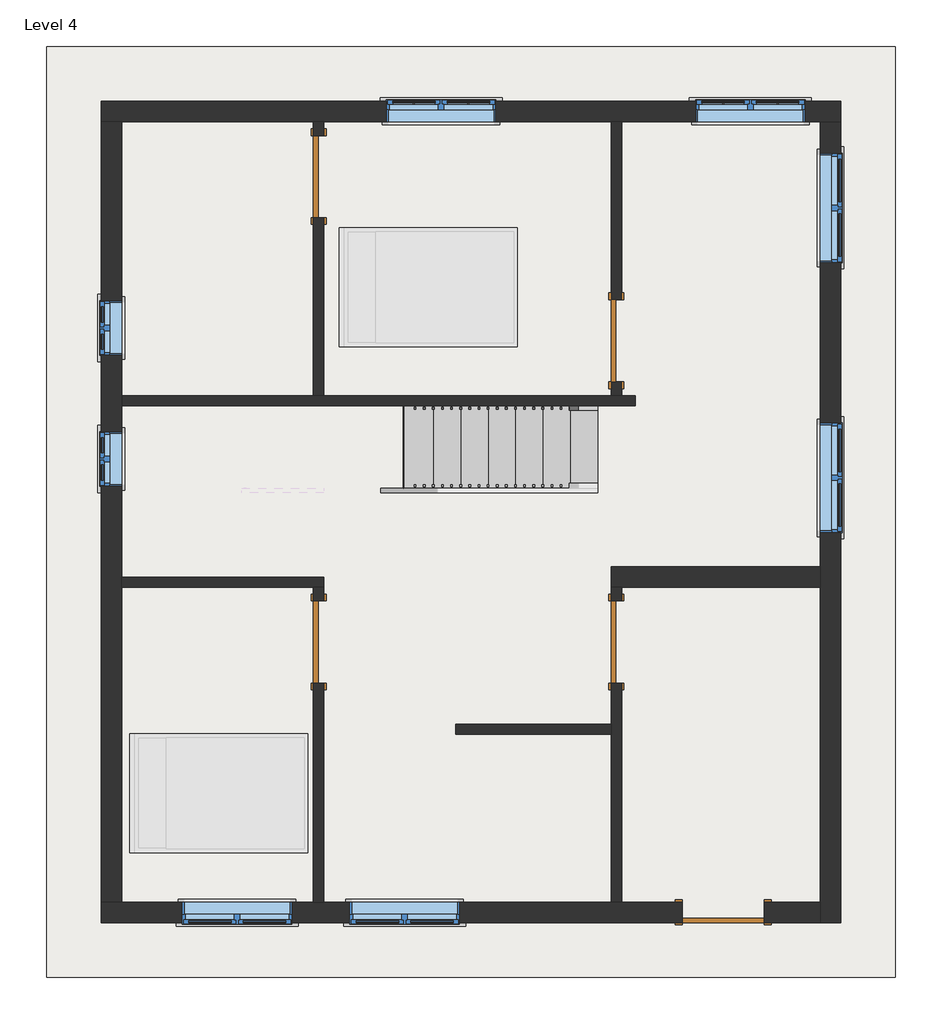
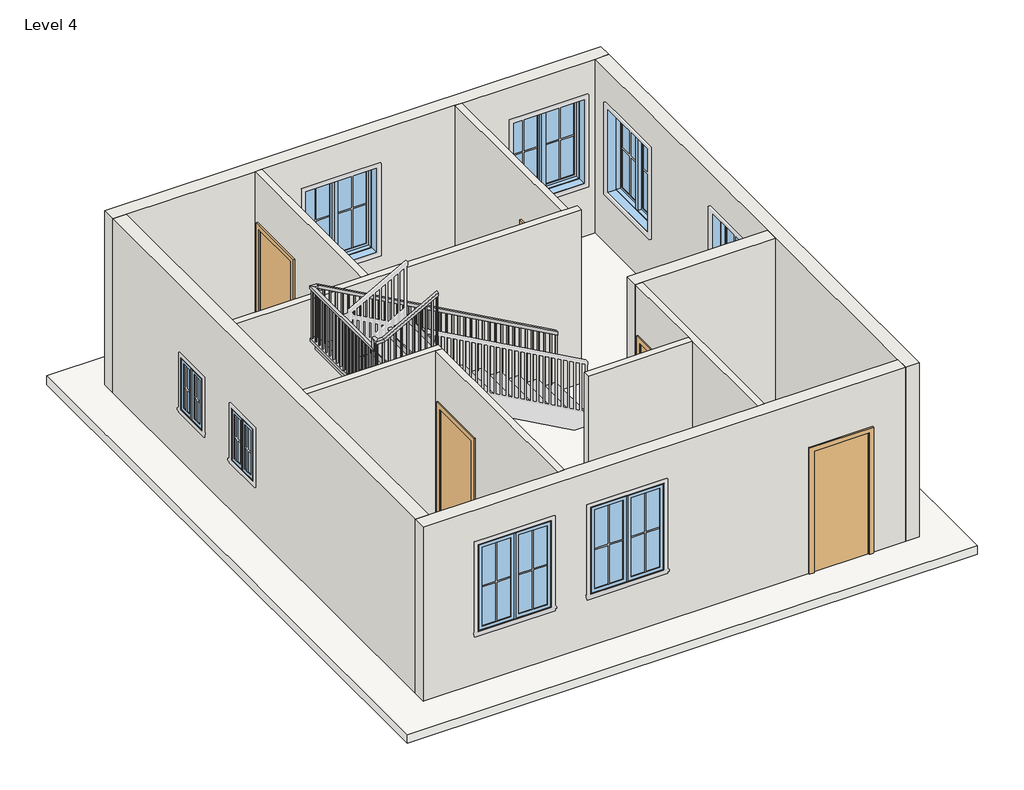
# One storey, part 1 of 2: 12 walls, 8 windows, 5 doors, 1 railing, 1 slab, 1 stair flight.
"""IFC4 building model written with IfcOpenShell, lengths in millimetres."""

from ifc_helpers import new_model, si_unit, frame, origin, place, context, project, spatial, polyline, outline, extrude, faceted_brep, transform, mapped, element, save
from components import door_e5f9f3c4, door_305aa2a5, door_0ca8825f, stair_flight_3eca97f2, window_c417fced, window_8377141f

model = new_model("IFC4")

# Units and contexts
model_context = context("Model", 3, world=origin())
ifc_project = project(units=[si_unit("LENGTHUNIT", "METRE", prefix="MILLI")], contexts=[model_context])

# Site, building, storey
site = spatial("IfcSite", under=ifc_project)
building = spatial("IfcBuilding", under=site)
storey = spatial("IfcBuildingStorey", under=building, Name="Level 4", Elevation=9144.0)

# Doors
placement = place(None, origin())
door_shape = door_e5f9f3c4(model_context)
element("IfcDoor", 1, ObjectType="Single-Flush : 36\" x 84\"", at=placement, inside=storey, context=model_context, shape_type="MappedRepresentation", body=[
    mapped(door_shape, transform((3689.35, 13938.7372886, 9144.0), x_axis=(0.0, 1.0, 0.0), y_axis=(-1.0, 0.0, 0.0), z_axis=(0.0, 0.0, 1.0))),
])
door_2_shape = door_305aa2a5(model_context)
element("IfcDoor", 2, ObjectType="Single-Flush : 36\" x 84\"", at=placement, inside=storey, context=model_context, shape_type="MappedRepresentation", body=[
    mapped(door_2_shape, transform((7004.05, 12109.9372886, 9144.0), x_axis=(0.0, -1.0, 0.0), y_axis=(1.0, 0.0, 0.0), z_axis=(0.0, 0.0, 1.0))),
])
element("IfcDoor", 3, ObjectType="Single-Flush : 36\" x 84\"", at=placement, inside=storey, context=model_context, shape_type="MappedRepresentation", body=[
    mapped(door_2_shape, transform((3689.3519847, 8757.1372886, 9144.0), x_axis=(0.0, -1.0, 0.0), y_axis=(1.0, 0.0, 0.0), z_axis=(0.0, 0.0, 1.0))),
])
element("IfcDoor", 4, ObjectType="Single-Flush : 36\" x 84\"", at=placement, inside=storey, context=model_context, shape_type="MappedRepresentation", body=[
    mapped(door_2_shape, transform((7004.05, 8757.1372886, 9144.0), x_axis=(0.0, -1.0, 0.0), y_axis=(1.0, 0.0, 0.0), z_axis=(0.0, 0.0, 1.0))),
])
door_3_shape = door_0ca8825f(model_context)
element("IfcDoor", 5, ObjectType="Single-Flush : 36\" x 84\"", at=placement, inside=storey, context=model_context, shape_type="MappedRepresentation", body=[
    mapped(door_3_shape, transform((8194.675, 5747.2372886, 9144.0), x_axis=(-1.0, 0.0, 0.0), y_axis=(0.0, -1.0, 0.0), z_axis=(0.0, 0.0, 1.0))),
])

# Railing
element("IfcRailing", 6, ObjectType="Handrail - Rectangular", at=placement, inside=storey, context=model_context, shape_type="SolidModel", body=[
    faceted_brep([(6794.5, 11335.2372886, 10227.7333333), (6794.5, 11335.2372886, 10169.620221), (6794.5, 11386.0372886, 10169.620221), (6794.5, 11386.0372886, 10227.7333333), (2832.1, 11335.2372886, 12429.0666667), (2818.9363978, 11335.2372886, 12378.2666667), (2818.9363978, 11386.0372886, 12378.2666667), (2832.1, 11386.0372886, 12429.0666667), (2768.6, 11335.2372886, 12429.0666667), (2768.6, 11335.2372886, 12378.2666667), (2717.8, 11386.0372886, 12378.2666667), (2717.8, 11386.0372886, 12429.0666667), (2768.6, 9608.0372886, 12429.0666667), (2768.6, 9557.2372886, 12378.2666667), (2717.8, 9557.2372886, 12378.2666667), (2717.8, 9608.0372886, 12429.0666667), (2768.6, 9608.0372886, 12605.4555402), (2768.6, 9557.2372886, 12554.6555402), (2717.8, 9557.2372886, 12554.6555402), (2717.8, 9608.0372886, 12605.4555402), (2768.6, 9531.8372886, 12605.4555402), (2768.6, 9531.8372886, 12554.6555402), (2717.8, 9481.0372886, 12554.6555402), (2717.8, 9481.0372886, 12605.4555402), (2844.8, 9531.8372886, 12605.4555402), (2857.9635773, 9531.8372886, 12554.6555402), (2857.9635773, 9481.0372886, 12554.6555402), (2844.8, 9481.0372886, 12605.4555402), (3746.5019847, 9531.8372886, 13106.4), (3746.5019847, 9481.0372886, 13106.4), (3746.5019847, 9481.0372886, 13048.2869174), (3746.5019847, 9531.8372886, 13048.2869174)], [[[0, 1, 2, 3]], [[1, 0, 4, 5]], [[2, 1, 5, 6]], [[3, 2, 6, 7]], [[0, 3, 7, 4]], [[5, 4, 8, 9]], [[6, 5, 9, 10]], [[7, 6, 10, 11]], [[4, 7, 11, 8]], [[9, 8, 12, 13]], [[10, 9, 13, 14]], [[11, 10, 14, 15]], [[8, 11, 15, 12]], [[13, 12, 16, 17]], [[14, 13, 17, 18]], [[15, 14, 18, 19]], [[12, 15, 19, 16]], [[17, 16, 20, 21]], [[18, 17, 21, 22]], [[19, 18, 22, 23]], [[16, 19, 23, 20]], [[21, 20, 24, 25]], [[22, 21, 25, 26]], [[23, 22, 26, 27]], [[20, 23, 27, 24]], [[28, 29, 30, 31]], [[25, 24, 28, 31]], [[26, 25, 31, 30]], [[27, 26, 30, 29]], [[24, 27, 29, 28]]]),
    extrude(outline(polyline([(13004.1894234, 3667.125), (12993.606113, 3648.075), (12022.6666667, 3648.075), (12022.6666667, 3667.125), (13004.1894234, 3667.125)])), frame((0.0, 9496.9122886, 0.0), z_axis=(0.0, 1.0, 0.0), x_axis=(0.0, 0.0, 1.0)), (0.0, 0.0, 1.0), 19.05),
    extrude(outline(polyline([(12947.7451014, 3565.525), (12937.1617911, 3546.475), (12022.6666667, 3546.475), (12022.6666667, 3565.525), (12947.7451014, 3565.525)])), frame((0.0, 9496.9122886, 0.0), z_axis=(0.0, 1.0, 0.0), x_axis=(0.0, 0.0, 1.0)), (0.0, 0.0, 1.0), 19.05),
    extrude(outline(polyline([(12891.3007795, 3463.925), (12880.7174691, 3444.875), (12022.6666667, 3444.875), (12022.6666667, 3463.925), (12891.3007795, 3463.925)])), frame((0.0, 9496.9122886, 0.0), z_axis=(0.0, 1.0, 0.0), x_axis=(0.0, 0.0, 1.0)), (0.0, 0.0, 1.0), 19.05),
    extrude(outline(polyline([(12834.85609, 3362.325), (12824.2727797, 3343.275), (11853.3333333, 3343.275), (11853.3333333, 3362.325), (12834.85609, 3362.325)])), frame((0.0, 9496.9122886, 0.0), z_axis=(0.0, 1.0, 0.0), x_axis=(0.0, 0.0, 1.0)), (0.0, 0.0, 1.0), 19.05),
    extrude(outline(polyline([(12778.4117681, 3260.725), (12767.8284577, 3241.675), (11853.3333333, 3241.675), (11853.3333333, 3260.725), (12778.4117681, 3260.725)])), frame((0.0, 9496.9122886, 0.0), z_axis=(0.0, 1.0, 0.0), x_axis=(0.0, 0.0, 1.0)), (0.0, 0.0, 1.0), 19.05),
    extrude(outline(polyline([(12721.9674462, 3159.125), (12711.3841358, 3140.075), (11853.3333333, 3140.075), (11853.3333333, 3159.125), (12721.9674462, 3159.125)])), frame((0.0, 9496.9122886, 0.0), z_axis=(0.0, 1.0, 0.0), x_axis=(0.0, 0.0, 1.0)), (0.0, 0.0, 1.0), 19.05),
    extrude(outline(polyline([(12665.5227567, 3057.525), (12654.9394463, 3038.475), (11684.0, 3038.475), (11684.0, 3057.525), (12665.5227567, 3057.525)])), frame((0.0, 9496.9122886, 0.0), z_axis=(0.0, 1.0, 0.0), x_axis=(0.0, 0.0, 1.0)), (0.0, 0.0, 1.0), 19.05),
    extrude(outline(polyline([(12609.0784348, 2955.925), (12598.4951244, 2936.875), (11684.0, 2936.875), (11684.0, 2955.925), (12609.0784348, 2955.925)])), frame((0.0, 9496.9122886, 0.0), z_axis=(0.0, 1.0, 0.0), x_axis=(0.0, 0.0, 1.0)), (0.0, 0.0, 1.0), 19.05),
    extrude(outline(polyline([(12552.6341128, 2854.325), (12542.0508025, 2835.275), (11684.0, 2835.275), (11684.0, 2854.325), (12552.6341128, 2854.325)])), frame((0.0, 9496.9122886, 0.0), z_axis=(0.0, 1.0, 0.0), x_axis=(0.0, 0.0, 1.0)), (0.0, 0.0, 1.0), 19.05),
    extrude(outline(polyline([(2733.675, 9541.3622886), (2752.725, 9541.3622886), (2752.725, 9522.3122886), (2733.675, 9522.3122886), (2733.675, 9541.3622886)])), frame((0.0, 0.0, 11514.6666667), z_axis=(0.0, 0.0, 1.0), x_axis=(1.0, 0.0, 0.0)), (0.0, 0.0, 1.0), 1039.9888736),
    extrude(outline(polyline([(2733.675, 9642.9622886), (2752.725, 9642.9622886), (2752.725, 9623.9122886), (2733.675, 9623.9122886), (2733.675, 9642.9622886)])), frame((0.0, 0.0, 11514.6666667), z_axis=(0.0, 0.0, 1.0), x_axis=(1.0, 0.0, 0.0)), (0.0, 0.0, 1.0), 863.6),
    extrude(outline(polyline([(2733.675, 9744.5622886), (2752.725, 9744.5622886), (2752.725, 9725.5122886), (2733.675, 9725.5122886), (2733.675, 9744.5622886)])), frame((0.0, 0.0, 11514.6666667), z_axis=(0.0, 0.0, 1.0), x_axis=(1.0, 0.0, 0.0)), (0.0, 0.0, 1.0), 863.6),
    extrude(outline(polyline([(2733.675, 9846.1622886), (2752.725, 9846.1622886), (2752.725, 9827.1122886), (2733.675, 9827.1122886), (2733.675, 9846.1622886)])), frame((0.0, 0.0, 11514.6666667), z_axis=(0.0, 0.0, 1.0), x_axis=(1.0, 0.0, 0.0)), (0.0, 0.0, 1.0), 863.6),
    extrude(outline(polyline([(2733.675, 9947.7622886), (2752.725, 9947.7622886), (2752.725, 9928.7122886), (2733.675, 9928.7122886), (2733.675, 9947.7622886)])), frame((0.0, 0.0, 11514.6666667), z_axis=(0.0, 0.0, 1.0), x_axis=(1.0, 0.0, 0.0)), (0.0, 0.0, 1.0), 863.6),
    extrude(outline(polyline([(2733.675, 10049.3622886), (2752.725, 10049.3622886), (2752.725, 10030.3122886), (2733.675, 10030.3122886), (2733.675, 10049.3622886)])), frame((0.0, 0.0, 11514.6666667), z_axis=(0.0, 0.0, 1.0), x_axis=(1.0, 0.0, 0.0)), (0.0, 0.0, 1.0), 863.6),
    extrude(outline(polyline([(2733.675, 10150.9622886), (2752.725, 10150.9622886), (2752.725, 10131.9122886), (2733.675, 10131.9122886), (2733.675, 10150.9622886)])), frame((0.0, 0.0, 11514.6666667), z_axis=(0.0, 0.0, 1.0), x_axis=(1.0, 0.0, 0.0)), (0.0, 0.0, 1.0), 863.6),
    extrude(outline(polyline([(2733.675, 10252.5622886), (2752.725, 10252.5622886), (2752.725, 10233.5122886), (2733.675, 10233.5122886), (2733.675, 10252.5622886)])), frame((0.0, 0.0, 11514.6666667), z_axis=(0.0, 0.0, 1.0), x_axis=(1.0, 0.0, 0.0)), (0.0, 0.0, 1.0), 863.6),
    extrude(outline(polyline([(2733.675, 10354.1622886), (2752.725, 10354.1622886), (2752.725, 10335.1122886), (2733.675, 10335.1122886), (2733.675, 10354.1622886)])), frame((0.0, 0.0, 11514.6666667), z_axis=(0.0, 0.0, 1.0), x_axis=(1.0, 0.0, 0.0)), (0.0, 0.0, 1.0), 863.6),
    extrude(outline(polyline([(2733.675, 10455.7622886), (2752.725, 10455.7622886), (2752.725, 10436.7122886), (2733.675, 10436.7122886), (2733.675, 10455.7622886)])), frame((0.0, 0.0, 11514.6666667), z_axis=(0.0, 0.0, 1.0), x_axis=(1.0, 0.0, 0.0)), (0.0, 0.0, 1.0), 863.6),
    extrude(outline(polyline([(2733.675, 10557.3622886), (2752.725, 10557.3622886), (2752.725, 10538.3122886), (2733.675, 10538.3122886), (2733.675, 10557.3622886)])), frame((0.0, 0.0, 11514.6666667), z_axis=(0.0, 0.0, 1.0), x_axis=(1.0, 0.0, 0.0)), (0.0, 0.0, 1.0), 863.6),
    extrude(outline(polyline([(2733.675, 10658.9622886), (2752.725, 10658.9622886), (2752.725, 10639.9122886), (2733.675, 10639.9122886), (2733.675, 10658.9622886)])), frame((0.0, 0.0, 11514.6666667), z_axis=(0.0, 0.0, 1.0), x_axis=(1.0, 0.0, 0.0)), (0.0, 0.0, 1.0), 863.6),
    extrude(outline(polyline([(2733.675, 10760.5622886), (2752.725, 10760.5622886), (2752.725, 10741.5122886), (2733.675, 10741.5122886), (2733.675, 10760.5622886)])), frame((0.0, 0.0, 11514.6666667), z_axis=(0.0, 0.0, 1.0), x_axis=(1.0, 0.0, 0.0)), (0.0, 0.0, 1.0), 863.6),
    extrude(outline(polyline([(2733.675, 10862.1622886), (2752.725, 10862.1622886), (2752.725, 10843.1122886), (2733.675, 10843.1122886), (2733.675, 10862.1622886)])), frame((0.0, 0.0, 11514.6666667), z_axis=(0.0, 0.0, 1.0), x_axis=(1.0, 0.0, 0.0)), (0.0, 0.0, 1.0), 863.6),
    extrude(outline(polyline([(2733.675, 10963.7622886), (2752.725, 10963.7622886), (2752.725, 10944.7122886), (2733.675, 10944.7122886), (2733.675, 10963.7622886)])), frame((0.0, 0.0, 11514.6666667), z_axis=(0.0, 0.0, 1.0), x_axis=(1.0, 0.0, 0.0)), (0.0, 0.0, 1.0), 863.6),
    extrude(outline(polyline([(2733.675, 11065.3622886), (2752.725, 11065.3622886), (2752.725, 11046.3122886), (2733.675, 11046.3122886), (2733.675, 11065.3622886)])), frame((0.0, 0.0, 11514.6666667), z_axis=(0.0, 0.0, 1.0), x_axis=(1.0, 0.0, 0.0)), (0.0, 0.0, 1.0), 863.6),
    extrude(outline(polyline([(2733.675, 11166.9622886), (2752.725, 11166.9622886), (2752.725, 11147.9122886), (2733.675, 11147.9122886), (2733.675, 11166.9622886)])), frame((0.0, 0.0, 11514.6666667), z_axis=(0.0, 0.0, 1.0), x_axis=(1.0, 0.0, 0.0)), (0.0, 0.0, 1.0), 863.6),
    extrude(outline(polyline([(2733.675, 11268.5622886), (2752.725, 11268.5622886), (2752.725, 11249.5122886), (2733.675, 11249.5122886), (2733.675, 11268.5622886)])), frame((0.0, 0.0, 11514.6666667), z_axis=(0.0, 0.0, 1.0), x_axis=(1.0, 0.0, 0.0)), (0.0, 0.0, 1.0), 863.6),
    extrude(outline(polyline([(12365.6618876, 2841.625), (12376.245221, 2822.575), (11514.6666667, 2822.575), (11514.6666667, 2841.625), (12365.6618876, 2841.625)])), frame((0.0, 11351.1122886, 0.0), z_axis=(0.0, 1.0, 0.0), x_axis=(0.0, 0.0, 1.0)), (0.0, 0.0, 1.0), 19.05),
    extrude(outline(polyline([(12309.2174432, 2943.225), (12319.8007765, 2924.175), (11345.3333333, 2924.175), (11345.3333333, 2943.225), (12309.2174432, 2943.225)])), frame((0.0, 11351.1122886, 0.0), z_axis=(0.0, 1.0, 0.0), x_axis=(0.0, 0.0, 1.0)), (0.0, 0.0, 1.0), 19.05),
    extrude(outline(polyline([(12252.7729988, 3044.825), (12263.3563321, 3025.775), (11345.3333333, 3025.775), (11345.3333333, 3044.825), (12252.7729988, 3044.825)])), frame((0.0, 11351.1122886, 0.0), z_axis=(0.0, 1.0, 0.0), x_axis=(0.0, 0.0, 1.0)), (0.0, 0.0, 1.0), 19.05),
    extrude(outline(polyline([(12196.3285543, 3146.425), (12206.9118876, 3127.375), (11345.3333333, 3127.375), (11345.3333333, 3146.425), (12196.3285543, 3146.425)])), frame((0.0, 11351.1122886, 0.0), z_axis=(0.0, 1.0, 0.0), x_axis=(0.0, 0.0, 1.0)), (0.0, 0.0, 1.0), 19.05),
    extrude(outline(polyline([(12139.8841099, 3248.025), (12150.4674432, 3228.975), (11176.0, 3228.975), (11176.0, 3248.025), (12139.8841099, 3248.025)])), frame((0.0, 11351.1122886, 0.0), z_axis=(0.0, 1.0, 0.0), x_axis=(0.0, 0.0, 1.0)), (0.0, 0.0, 1.0), 19.05),
    extrude(outline(polyline([(12083.4396654, 3349.625), (12094.0229988, 3330.575), (11176.0, 3330.575), (11176.0, 3349.625), (12083.4396654, 3349.625)])), frame((0.0, 11351.1122886, 0.0), z_axis=(0.0, 1.0, 0.0), x_axis=(0.0, 0.0, 1.0)), (0.0, 0.0, 1.0), 19.05),
    extrude(outline(polyline([(12026.995221, 3451.225), (12037.5785543, 3432.175), (11176.0, 3432.175), (11176.0, 3451.225), (12026.995221, 3451.225)])), frame((0.0, 11351.1122886, 0.0), z_axis=(0.0, 1.0, 0.0), x_axis=(0.0, 0.0, 1.0)), (0.0, 0.0, 1.0), 19.05),
    extrude(outline(polyline([(11970.5507765, 3552.825), (11981.1341099, 3533.775), (11006.6666667, 3533.775), (11006.6666667, 3552.825), (11970.5507765, 3552.825)])), frame((0.0, 11351.1122886, 0.0), z_axis=(0.0, 1.0, 0.0), x_axis=(0.0, 0.0, 1.0)), (0.0, 0.0, 1.0), 19.05),
    extrude(outline(polyline([(11914.1063321, 3654.425), (11924.6896654, 3635.375), (11006.6666667, 3635.375), (11006.6666667, 3654.425), (11914.1063321, 3654.425)])), frame((0.0, 11351.1122886, 0.0), z_axis=(0.0, 1.0, 0.0), x_axis=(0.0, 0.0, 1.0)), (0.0, 0.0, 1.0), 19.05),
    extrude(outline(polyline([(11857.6618876, 3756.025), (11868.245221, 3736.975), (11006.6666667, 3736.975), (11006.6666667, 3756.025), (11857.6618876, 3756.025)])), frame((0.0, 11351.1122886, 0.0), z_axis=(0.0, 1.0, 0.0), x_axis=(0.0, 0.0, 1.0)), (0.0, 0.0, 1.0), 19.05),
    extrude(outline(polyline([(11801.2174432, 3857.625), (11811.8007765, 3838.575), (10837.3333333, 3838.575), (10837.3333333, 3857.625), (11801.2174432, 3857.625)])), frame((0.0, 11351.1122886, 0.0), z_axis=(0.0, 1.0, 0.0), x_axis=(0.0, 0.0, 1.0)), (0.0, 0.0, 1.0), 19.05),
    extrude(outline(polyline([(11744.7729988, 3959.225), (11755.3563321, 3940.175), (10837.3333333, 3940.175), (10837.3333333, 3959.225), (11744.7729988, 3959.225)])), frame((0.0, 11351.1122886, 0.0), z_axis=(0.0, 1.0, 0.0), x_axis=(0.0, 0.0, 1.0)), (0.0, 0.0, 1.0), 19.05),
    extrude(outline(polyline([(11688.3285543, 4060.825), (11698.9118876, 4041.775), (10837.3333333, 4041.775), (10837.3333333, 4060.825), (11688.3285543, 4060.825)])), frame((0.0, 11351.1122886, 0.0), z_axis=(0.0, 1.0, 0.0), x_axis=(0.0, 0.0, 1.0)), (0.0, 0.0, 1.0), 19.05),
    extrude(outline(polyline([(11631.8841099, 4162.425), (11642.4674432, 4143.375), (10668.0, 4143.375), (10668.0, 4162.425), (11631.8841099, 4162.425)])), frame((0.0, 11351.1122886, 0.0), z_axis=(0.0, 1.0, 0.0), x_axis=(0.0, 0.0, 1.0)), (0.0, 0.0, 1.0), 19.05),
    extrude(outline(polyline([(11575.4396654, 4264.025), (11586.0229988, 4244.975), (10668.0, 4244.975), (10668.0, 4264.025), (11575.4396654, 4264.025)])), frame((0.0, 11351.1122886, 0.0), z_axis=(0.0, 1.0, 0.0), x_axis=(0.0, 0.0, 1.0)), (0.0, 0.0, 1.0), 19.05),
    extrude(outline(polyline([(11518.995221, 4365.625), (11529.5785543, 4346.575), (10668.0, 4346.575), (10668.0, 4365.625), (11518.995221, 4365.625)])), frame((0.0, 11351.1122886, 0.0), z_axis=(0.0, 1.0, 0.0), x_axis=(0.0, 0.0, 1.0)), (0.0, 0.0, 1.0), 19.05),
    extrude(outline(polyline([(11462.5507765, 4467.225), (11473.1341099, 4448.175), (10498.6666667, 4448.175), (10498.6666667, 4467.225), (11462.5507765, 4467.225)])), frame((0.0, 11351.1122886, 0.0), z_axis=(0.0, 1.0, 0.0), x_axis=(0.0, 0.0, 1.0)), (0.0, 0.0, 1.0), 19.05),
    extrude(outline(polyline([(11406.1063321, 4568.825), (11416.6896654, 4549.775), (10498.6666667, 4549.775), (10498.6666667, 4568.825), (11406.1063321, 4568.825)])), frame((0.0, 11351.1122886, 0.0), z_axis=(0.0, 1.0, 0.0), x_axis=(0.0, 0.0, 1.0)), (0.0, 0.0, 1.0), 19.05),
    extrude(outline(polyline([(11349.6618876, 4670.425), (11360.245221, 4651.375), (10498.6666667, 4651.375), (10498.6666667, 4670.425), (11349.6618876, 4670.425)])), frame((0.0, 11351.1122886, 0.0), z_axis=(0.0, 1.0, 0.0), x_axis=(0.0, 0.0, 1.0)), (0.0, 0.0, 1.0), 19.05),
    extrude(outline(polyline([(11293.2174432, 4772.025), (11303.8007765, 4752.975), (10329.3333333, 4752.975), (10329.3333333, 4772.025), (11293.2174432, 4772.025)])), frame((0.0, 11351.1122886, 0.0), z_axis=(0.0, 1.0, 0.0), x_axis=(0.0, 0.0, 1.0)), (0.0, 0.0, 1.0), 19.05),
    extrude(outline(polyline([(11236.7729988, 4873.625), (11247.3563321, 4854.575), (10329.3333333, 4854.575), (10329.3333333, 4873.625), (11236.7729988, 4873.625)])), frame((0.0, 11351.1122886, 0.0), z_axis=(0.0, 1.0, 0.0), x_axis=(0.0, 0.0, 1.0)), (0.0, 0.0, 1.0), 19.05),
    extrude(outline(polyline([(11180.3285543, 4975.225), (11190.9118876, 4956.175), (10329.3333333, 4956.175), (10329.3333333, 4975.225), (11180.3285543, 4975.225)])), frame((0.0, 11351.1122886, 0.0), z_axis=(0.0, 1.0, 0.0), x_axis=(0.0, 0.0, 1.0)), (0.0, 0.0, 1.0), 19.05),
    extrude(outline(polyline([(11123.8841099, 5076.825), (11134.4674432, 5057.775), (10160.0, 5057.775), (10160.0, 5076.825), (11123.8841099, 5076.825)])), frame((0.0, 11351.1122886, 0.0), z_axis=(0.0, 1.0, 0.0), x_axis=(0.0, 0.0, 1.0)), (0.0, 0.0, 1.0), 19.05),
    extrude(outline(polyline([(11067.4396654, 5178.425), (11078.0229988, 5159.375), (10160.0, 5159.375), (10160.0, 5178.425), (11067.4396654, 5178.425)])), frame((0.0, 11351.1122886, 0.0), z_axis=(0.0, 1.0, 0.0), x_axis=(0.0, 0.0, 1.0)), (0.0, 0.0, 1.0), 19.05),
    extrude(outline(polyline([(11010.995221, 5280.025), (11021.5785543, 5260.975), (10160.0, 5260.975), (10160.0, 5280.025), (11010.995221, 5280.025)])), frame((0.0, 11351.1122886, 0.0), z_axis=(0.0, 1.0, 0.0), x_axis=(0.0, 0.0, 1.0)), (0.0, 0.0, 1.0), 19.05),
    extrude(outline(polyline([(10954.5507765, 5381.625), (10965.1341099, 5362.575), (9990.6666667, 5362.575), (9990.6666667, 5381.625), (10954.5507765, 5381.625)])), frame((0.0, 11351.1122886, 0.0), z_axis=(0.0, 1.0, 0.0), x_axis=(0.0, 0.0, 1.0)), (0.0, 0.0, 1.0), 19.05),
    extrude(outline(polyline([(10898.1063321, 5483.225), (10908.6896654, 5464.175), (9990.6666667, 5464.175), (9990.6666667, 5483.225), (10898.1063321, 5483.225)])), frame((0.0, 11351.1122886, 0.0), z_axis=(0.0, 1.0, 0.0), x_axis=(0.0, 0.0, 1.0)), (0.0, 0.0, 1.0), 19.05),
    extrude(outline(polyline([(10841.6618876, 5584.825), (10852.245221, 5565.775), (9990.6666667, 5565.775), (9990.6666667, 5584.825), (10841.6618876, 5584.825)])), frame((0.0, 11351.1122886, 0.0), z_axis=(0.0, 1.0, 0.0), x_axis=(0.0, 0.0, 1.0)), (0.0, 0.0, 1.0), 19.05),
    extrude(outline(polyline([(10785.2174432, 5686.425), (10795.8007765, 5667.375), (9821.3333333, 5667.375), (9821.3333333, 5686.425), (10785.2174432, 5686.425)])), frame((0.0, 11351.1122886, 0.0), z_axis=(0.0, 1.0, 0.0), x_axis=(0.0, 0.0, 1.0)), (0.0, 0.0, 1.0), 19.05),
    extrude(outline(polyline([(10728.7729988, 5788.025), (10739.3563321, 5768.975), (9821.3333333, 5768.975), (9821.3333333, 5788.025), (10728.7729988, 5788.025)])), frame((0.0, 11351.1122886, 0.0), z_axis=(0.0, 1.0, 0.0), x_axis=(0.0, 0.0, 1.0)), (0.0, 0.0, 1.0), 19.05),
    extrude(outline(polyline([(10672.3285543, 5889.625), (10682.9118876, 5870.575), (9821.3333333, 5870.575), (9821.3333333, 5889.625), (10672.3285543, 5889.625)])), frame((0.0, 11351.1122886, 0.0), z_axis=(0.0, 1.0, 0.0), x_axis=(0.0, 0.0, 1.0)), (0.0, 0.0, 1.0), 19.05),
    extrude(outline(polyline([(10615.8841099, 5991.225), (10626.4674432, 5972.175), (9652.0, 5972.175), (9652.0, 5991.225), (10615.8841099, 5991.225)])), frame((0.0, 11351.1122886, 0.0), z_axis=(0.0, 1.0, 0.0), x_axis=(0.0, 0.0, 1.0)), (0.0, 0.0, 1.0), 19.05),
    extrude(outline(polyline([(10559.4396654, 6092.825), (10570.0229988, 6073.775), (9652.0, 6073.775), (9652.0, 6092.825), (10559.4396654, 6092.825)])), frame((0.0, 11351.1122886, 0.0), z_axis=(0.0, 1.0, 0.0), x_axis=(0.0, 0.0, 1.0)), (0.0, 0.0, 1.0), 19.05),
    extrude(outline(polyline([(10502.995221, 6194.425), (10513.5785543, 6175.375), (9652.0, 6175.375), (9652.0, 6194.425), (10502.995221, 6194.425)])), frame((0.0, 11351.1122886, 0.0), z_axis=(0.0, 1.0, 0.0), x_axis=(0.0, 0.0, 1.0)), (0.0, 0.0, 1.0), 19.05),
    extrude(outline(polyline([(10446.5507765, 6296.025), (10457.1341099, 6276.975), (9482.6666667, 6276.975), (9482.6666667, 6296.025), (10446.5507765, 6296.025)])), frame((0.0, 11351.1122886, 0.0), z_axis=(0.0, 1.0, 0.0), x_axis=(0.0, 0.0, 1.0)), (0.0, 0.0, 1.0), 19.05),
    extrude(outline(polyline([(10390.1063321, 6397.625), (10400.6896654, 6378.575), (9482.6666667, 6378.575), (9482.6666667, 6397.625), (10390.1063321, 6397.625)])), frame((0.0, 11351.1122886, 0.0), z_axis=(0.0, 1.0, 0.0), x_axis=(0.0, 0.0, 1.0)), (0.0, 0.0, 1.0), 19.05),
    extrude(outline(polyline([(10333.6618876, 6499.225), (10344.245221, 6480.175), (9482.6666667, 6480.175), (9482.6666667, 6499.225), (10333.6618876, 6499.225)])), frame((0.0, 11351.1122886, 0.0), z_axis=(0.0, 1.0, 0.0), x_axis=(0.0, 0.0, 1.0)), (0.0, 0.0, 1.0), 19.05),
    extrude(outline(polyline([(10277.2174432, 6600.825), (10287.8007765, 6581.775), (9313.3333333, 6581.775), (9313.3333333, 6600.825), (10277.2174432, 6600.825)])), frame((0.0, 11351.1122886, 0.0), z_axis=(0.0, 1.0, 0.0), x_axis=(0.0, 0.0, 1.0)), (0.0, 0.0, 1.0), 19.05),
    extrude(outline(polyline([(10220.7729988, 6702.425), (10231.3563321, 6683.375), (9313.3333333, 6683.375), (9313.3333333, 6702.425), (10220.7729988, 6702.425)])), frame((0.0, 11351.1122886, 0.0), z_axis=(0.0, 1.0, 0.0), x_axis=(0.0, 0.0, 1.0)), (0.0, 0.0, 1.0), 19.05),
    extrude(outline(polyline([(2733.675, 9515.9622886), (2752.725, 9515.9622886), (2752.725, 9496.9122886), (2733.675, 9496.9122886), (2733.675, 9515.9622886)])), frame((0.0, 0.0, 11514.6666667), z_axis=(0.0, 0.0, 1.0), x_axis=(1.0, 0.0, 0.0)), (0.0, 0.0, 1.0), 1039.9888736),
    extrude(outline(polyline([(2752.725, 11370.1622886), (2752.725, 11351.1122886), (2733.675, 11351.1122886), (2733.675, 11370.1622886), (2752.725, 11370.1622886)])), frame((0.0, 0.0, 11514.6666667), z_axis=(0.0, 0.0, 1.0), x_axis=(1.0, 0.0, 0.0)), (0.0, 0.0, 1.0), 863.6),
    extrude(outline(polyline([(13048.2869174, 3746.5019847), (13037.703607, 3727.4519847), (12022.6666667, 3727.4519847), (12022.6666667, 3746.5019847), (13048.2869174, 3746.5019847)])), frame((0.0, 9496.9122886, 0.0), z_axis=(0.0, 1.0, 0.0), x_axis=(0.0, 0.0, 1.0)), (0.0, 0.0, 1.0), 19.05),
    extrude(outline(polyline([(10169.620221, 6794.5), (10180.2035543, 6775.45), (9313.3333333, 6775.45), (9313.3333333, 6794.5), (10169.620221, 6794.5)])), frame((0.0, 11351.1122886, 0.0), z_axis=(0.0, 1.0, 0.0), x_axis=(0.0, 0.0, 1.0)), (0.0, 0.0, 1.0), 19.05),
])

# Slab
element("IfcSlab", 7, ObjectType="Generic - 12\"", at=placement, inside=storey, context=model_context, shape_type="SweptSolid", body=[
    extrude(outline(polyline([(10109.2, 15386.5372886), (10109.2, 5023.3372886), (660.4, 5023.3372886), (660.4, 15386.5372886), (10109.2, 15386.5372886)])), frame((0.0, 0.0, 8991.6), z_axis=(0.0, 0.0, 1.0), x_axis=(1.0, 0.0, 0.0)), (0.0, 0.0, 1.0), 152.4),
])

# Stair flight
stair_flight_shape = stair_flight_3eca97f2(model_context)
element("IfcStairFlight", 8, ObjectType="2\" Tread 1\" Nosing 1/4\" Riser", at=placement, inside=storey, context=model_context, shape_type="MappedRepresentation", body=[
    mapped(stair_flight_shape, transform((0.0, 0.0, 0.0), x_axis=(1.0, 0.0, 0.0), y_axis=(0.0, 1.0, 0.0), z_axis=(0.0, 0.0, 1.0))),
])

# Walls
element("IfcWall", 9, ObjectType="Generic - 5\"", at=placement, inside=storey, context=model_context, shape_type="SweptSolid", body=[
    extrude(outline(polyline([(14548.3372886, 9144.0), (14395.9372886, 9144.0), (14395.9372886, 11277.6), (13481.5372886, 11277.6), (13481.5372886, 9144.0), (11500.3372886, 9144.0), (11500.3372886, 12192.0), (14548.3372886, 12192.0), (14548.3372886, 9144.0)])), frame((3632.2, 0.0, 0.0), z_axis=(1.0, 0.0, 0.0), x_axis=(0.0, 1.0, 0.0)), (0.0, 0.0, 1.0), 114.3),
])
element("IfcWall", 10, ObjectType="Generic - 5\"", at=placement, inside=storey, context=model_context, shape_type="SweptSolid", body=[
    extrude(outline(polyline([(11652.7372886, 11277.6), (11652.7372886, 9144.0), (11500.3372886, 9144.0), (11500.3372886, 12192.0), (14548.3372886, 12192.0), (14548.3372886, 9144.0), (12567.1372886, 9144.0), (12567.1372886, 11277.6), (11652.7372886, 11277.6)])), frame((6946.9, 0.0, 0.0), z_axis=(1.0, 0.0, 0.0), x_axis=(0.0, 1.0, 0.0)), (0.0, 0.0, 1.0), 114.3),
])
element("IfcWall", 11, ObjectType="Generic - 5\"", at=placement, inside=storey, context=model_context, shape_type="Brep", body=[
    faceted_brep([(1498.6, 11386.0372886, 9144.0), (7213.6, 11386.0372886, 9144.0), (7213.6, 11386.0372886, 12192.0), (1498.6, 11386.0372886, 12192.0), (1498.6, 11500.3372886, 9144.0), (1498.6, 11500.3372886, 12192.0), (3632.2, 11500.3372886, 12192.0), (3746.5, 11500.3372886, 12192.0), (6946.9, 11500.3372886, 12192.0), (7061.2, 11500.3372886, 12192.0), (7213.6, 11500.3372886, 12192.0), (7213.6, 11500.3372886, 9144.0), (7061.2, 11500.3372886, 9144.0), (6946.9, 11500.3372886, 9144.0), (3746.5, 11500.3372886, 9144.0), (3632.2, 11500.3372886, 9144.0)], [[[0, 1, 2, 3]], [[4, 5, 6, 7, 8, 9, 10, 11, 12, 13, 14, 15]], [[1, 0, 4, 15, 14, 13, 12, 11]], [[2, 1, 11, 10]], [[3, 2, 10, 9, 8, 7, 6, 5]], [[0, 3, 5, 4]]]),
])
element("IfcWall", 12, ObjectType="Generic - 5\"", at=placement, inside=storey, context=model_context, shape_type="Brep", body=[
    faceted_brep([(1498.6, 9366.7372886, 9144.0), (3632.2019847, 9366.7372886, 9144.0), (3746.5019847, 9366.7372886, 9144.0), (3746.5019847, 9366.7372886, 12192.0), (3632.2019847, 9366.7372886, 12192.0), (1498.6, 9366.7372886, 12192.0), (1498.6, 9481.0372886, 9144.0), (1498.6, 9481.0372886, 12192.0), (3746.5019847, 9481.0372886, 12192.0), (3746.5019847, 9481.0372886, 9144.0)], [[[0, 1, 2, 3, 4, 5]], [[6, 7, 8, 9]], [[2, 1, 0, 6, 9]], [[5, 4, 3, 8, 7]], [[0, 5, 7, 6]], [[3, 2, 9, 8]]]),
])
element("IfcWall", 13, ObjectType="Generic - 5\"", at=placement, inside=storey, context=model_context, shape_type="SweptSolid", body=[
    extrude(outline(polyline([(8299.9372886, 11277.6), (8299.9372886, 9144.0), (5861.5372886, 9144.0), (5861.5372886, 12192.0), (9366.7372886, 12192.0), (9366.7372886, 9144.0), (9214.3372886, 9144.0), (9214.3372886, 11277.6), (8299.9372886, 11277.6)])), frame((3632.2019847, 0.0, 0.0), z_axis=(1.0, 0.0, 0.0), x_axis=(0.0, 1.0, 0.0)), (0.0, 0.0, 1.0), 114.3),
])
element("IfcWall", 14, ObjectType="Generic - 5\"", at=placement, inside=storey, context=model_context, shape_type="Brep", body=[
    faceted_brep([(7061.2, 5861.5372886, 9144.0), (7061.2, 8299.9372886, 9144.0), (7061.2, 8299.9372886, 11277.6), (7061.2, 9214.3372886, 11277.6), (7061.2, 9214.3372886, 9144.0), (7061.2, 9366.7372886, 9144.0), (7061.2, 9366.7372886, 12192.0), (7061.2, 5861.5372886, 12192.0), (6946.9, 8299.9372886, 11277.6), (6946.9, 8299.9372886, 9144.0), (6946.9, 7842.7372886, 9144.0), (6946.9, 7728.4372886, 9144.0), (6946.9, 5861.5372886, 9144.0), (6946.9, 5861.5372886, 12192.0), (6946.9, 7728.4372886, 12192.0), (6946.9, 7842.7372886, 12192.0), (6946.9, 9366.7372886, 12192.0), (6946.9, 9366.7372886, 9144.0), (6946.9, 9214.3372886, 9144.0), (6946.9, 9214.3372886, 11277.6)], [[[0, 1, 2, 3, 4, 5, 6, 7]], [[8, 9, 10, 11, 12, 13, 14, 15, 16, 17, 18, 19]], [[18, 17, 5, 4]], [[12, 11, 10, 9, 1, 0]], [[7, 6, 16, 15, 14, 13]], [[0, 7, 13, 12]], [[6, 5, 17, 16]], [[2, 1, 9, 8]], [[3, 2, 8, 19]], [[4, 3, 19, 18]]]),
])
element("IfcWall", 15, ObjectType="Generic - 5\"", at=placement, inside=storey, context=model_context, shape_type="SweptSolid", body=[
    extrude(outline(polyline([(5215.2207778, 7842.7372886), (6946.9, 7842.7372886), (6946.9, 7728.4372886), (5215.2207778, 7728.4372886), (5215.2207778, 7842.7372886)])), frame((0.0, 0.0, 9144.0), z_axis=(0.0, 0.0, 1.0), x_axis=(1.0, 0.0, 0.0)), (0.0, 0.0, 1.0), 3048.0),
])
element("IfcWall", 16, ObjectType="Generic - 8\"", at=placement, inside=storey, context=model_context, shape_type="Brep", body=[
    faceted_brep([(1270.0, 14548.3372886, 9144.0), (1498.6, 14548.3372886, 9144.0), (3632.2, 14548.3372886, 9144.0), (3746.5, 14548.3372886, 9144.0), (6946.9, 14548.3372886, 9144.0), (7061.2, 14548.3372886, 9144.0), (9271.0, 14548.3372886, 9144.0), (9499.6, 14548.3372886, 9144.0), (9499.6, 14548.3372886, 12192.0), (9271.0, 14548.3372886, 12192.0), (7061.2, 14548.3372886, 12192.0), (6946.9, 14548.3372886, 12192.0), (3746.5, 14548.3372886, 12192.0), (3632.2, 14548.3372886, 12192.0), (1498.6, 14548.3372886, 12192.0), (1270.0, 14548.3372886, 12192.0), (9105.9, 14548.3372886, 11582.4), (9105.9, 14548.3372886, 10058.4), (7886.7, 14548.3372886, 10058.4), (7886.7, 14548.3372886, 11582.4), (5662.6125, 14548.3372886, 11582.4), (5662.6125, 14548.3372886, 10058.4), (4443.4125, 14548.3372886, 10058.4), (4443.4125, 14548.3372886, 11582.4), (1270.0, 14776.9372886, 9144.0), (1270.0, 14776.9372886, 12192.0), (9499.6, 14776.9372886, 12192.0), (9499.6, 14776.9372886, 9144.0), (9105.9, 14776.9372886, 11582.4), (7886.7, 14776.9372886, 11582.4), (7886.7, 14776.9372886, 10058.4), (9105.9, 14776.9372886, 10058.4), (5662.6125, 14776.9372886, 11582.4), (4443.4125, 14776.9372886, 11582.4), (4443.4125, 14776.9372886, 10058.4), (5662.6125, 14776.9372886, 10058.4)], [[[0, 1, 2, 3, 4, 5, 6, 7, 8, 9, 10, 11, 12, 13, 14, 15], [16, 17, 18, 19], [20, 21, 22, 23]], [[24, 25, 26, 27], [28, 29, 30, 31], [32, 33, 34, 35]], [[7, 6, 5, 4, 3, 2, 1, 0, 24, 27]], [[15, 14, 13, 12, 11, 10, 9, 8, 26, 25]], [[8, 7, 27, 26]], [[0, 15, 25, 24]], [[17, 16, 28, 31]], [[18, 17, 31, 30]], [[19, 18, 30, 29]], [[16, 19, 29, 28]], [[21, 20, 32, 35]], [[22, 21, 35, 34]], [[23, 22, 34, 33]], [[20, 23, 33, 32]]]),
])
element("IfcWall", 17, ObjectType="Generic - 8\"", at=placement, inside=storey, context=model_context, shape_type="Brep", body=[
    faceted_brep([(9271.0, 14548.3372886, 9144.0), (9271.0, 9595.3372886, 9144.0), (9271.0, 9366.7372886, 9144.0), (9271.0, 5861.5372886, 9144.0), (9271.0, 5632.9372886, 9144.0), (9271.0, 5632.9372886, 12192.0), (9271.0, 5861.5372886, 12192.0), (9271.0, 9366.7372886, 12192.0), (9271.0, 9595.3372886, 12192.0), (9271.0, 14548.3372886, 12192.0), (9271.0, 12979.8872886, 11582.4), (9271.0, 12979.8872886, 10058.4), (9271.0, 14199.0872886, 10058.4), (9271.0, 14199.0872886, 11582.4), (9271.0, 9976.3372886, 11582.4), (9271.0, 9976.3372886, 10058.4), (9271.0, 11195.5372886, 10058.4), (9271.0, 11195.5372886, 11582.4), (9499.6, 14548.3372886, 9144.0), (9499.6, 14548.3372886, 12192.0), (9499.6, 5632.9372886, 12192.0), (9499.6, 5632.9372886, 9144.0), (9499.6, 12979.8872886, 11582.4), (9499.6, 14199.0872886, 11582.4), (9499.6, 14199.0872886, 10058.4), (9499.6, 12979.8872886, 10058.4), (9499.6, 9976.3372886, 11582.4), (9499.6, 11195.5372886, 11582.4), (9499.6, 11195.5372886, 10058.4), (9499.6, 9976.3372886, 10058.4)], [[[0, 1, 2, 3, 4, 5, 6, 7, 8, 9], [10, 11, 12, 13], [14, 15, 16, 17]], [[18, 19, 20, 21], [22, 23, 24, 25], [26, 27, 28, 29]], [[4, 3, 2, 1, 0, 18, 21]], [[9, 8, 7, 6, 5, 20, 19]], [[0, 9, 19, 18]], [[5, 4, 21, 20]], [[11, 10, 22, 25]], [[12, 11, 25, 24]], [[13, 12, 24, 23]], [[10, 13, 23, 22]], [[15, 14, 26, 29]], [[16, 15, 29, 28]], [[17, 16, 28, 27]], [[14, 17, 27, 26]]]),
])
element("IfcWall", 18, ObjectType="Generic - 8\"", at=placement, inside=storey, context=model_context, shape_type="Brep", body=[
    faceted_brep([(7737.475, 5861.5372886, 11277.6), (7737.475, 5861.5372886, 9144.0), (7061.2, 5861.5372886, 9144.0), (6946.9, 5861.5372886, 9144.0), (3746.5019847, 5861.5372886, 9144.0), (3632.2019847, 5861.5372886, 9144.0), (1498.6, 5861.5372886, 9144.0), (1270.0, 5861.5372886, 9144.0), (1270.0, 5861.5372886, 12192.0), (1498.6, 5861.5372886, 12192.0), (3632.2019847, 5861.5372886, 12192.0), (3746.5019847, 5861.5372886, 12192.0), (6946.9, 5861.5372886, 12192.0), (7061.2, 5861.5372886, 12192.0), (9271.0, 5861.5372886, 12192.0), (9271.0, 5861.5372886, 9144.0), (8651.875, 5861.5372886, 9144.0), (8651.875, 5861.5372886, 11277.6), (4037.8082347, 5861.5372886, 11582.4), (4037.8082347, 5861.5372886, 10058.4), (5257.0082347, 5861.5372886, 10058.4), (5257.0082347, 5861.5372886, 11582.4), (2173.2894847, 5861.5372886, 11582.4), (2173.2894847, 5861.5372886, 10058.4), (3392.4894847, 5861.5372886, 10058.4), (3392.4894847, 5861.5372886, 11582.4), (1270.0, 5632.9372886, 9144.0), (7737.475, 5632.9372886, 9144.0), (7737.475, 5632.9372886, 11277.6), (8651.875, 5632.9372886, 11277.6), (8651.875, 5632.9372886, 9144.0), (9271.0, 5632.9372886, 9144.0), (9271.0, 5632.9372886, 12192.0), (1270.0, 5632.9372886, 12192.0), (4037.8082347, 5632.9372886, 11582.4), (5257.0082347, 5632.9372886, 11582.4), (5257.0082347, 5632.9372886, 10058.4), (4037.8082347, 5632.9372886, 10058.4), (2173.2894847, 5632.9372886, 11582.4), (3392.4894847, 5632.9372886, 11582.4), (3392.4894847, 5632.9372886, 10058.4), (2173.2894847, 5632.9372886, 10058.4)], [[[0, 1, 2, 3, 4, 5, 6, 7, 8, 9, 10, 11, 12, 13, 14, 15, 16, 17], [18, 19, 20, 21], [22, 23, 24, 25]], [[26, 27, 28, 29, 30, 31, 32, 33], [34, 35, 36, 37], [38, 39, 40, 41]], [[16, 15, 31, 30]], [[7, 6, 5, 4, 3, 2, 1, 27, 26]], [[14, 13, 12, 11, 10, 9, 8, 33, 32]], [[15, 14, 32, 31]], [[8, 7, 26, 33]], [[19, 18, 34, 37]], [[20, 19, 37, 36]], [[21, 20, 36, 35]], [[18, 21, 35, 34]], [[23, 22, 38, 41]], [[24, 23, 41, 40]], [[25, 24, 40, 39]], [[22, 25, 39, 38]], [[28, 27, 1, 0]], [[29, 28, 0, 17]], [[30, 29, 17, 16]]]),
])
element("IfcWall", 19, ObjectType="Generic - 8\"", at=placement, inside=storey, context=model_context, shape_type="Brep", body=[
    faceted_brep([(1498.6, 5861.5372886, 9144.0), (1498.6, 9366.7372886, 9144.0), (1498.6, 9481.0372886, 9144.0), (1498.6, 11386.0372886, 9144.0), (1498.6, 11500.3372886, 9144.0), (1498.6, 14548.3372886, 9144.0), (1498.6, 14548.3372886, 12192.0), (1498.6, 11500.3372886, 12192.0), (1498.6, 11386.0372886, 12192.0), (1498.6, 9481.0372886, 12192.0), (1498.6, 9366.7372886, 12192.0), (1498.6, 5861.5372886, 12192.0), (1498.6, 12557.6122886, 10972.8), (1498.6, 12557.6122886, 10058.4), (1498.6, 11948.0122886, 10058.4), (1498.6, 11948.0122886, 10972.8), (1498.6, 11100.2872886, 10972.8), (1498.6, 11100.2872886, 10058.4), (1498.6, 10490.6872886, 10058.4), (1498.6, 10490.6872886, 10972.8), (1270.0, 5861.5372886, 9144.0), (1270.0, 5861.5372886, 12192.0), (1270.0, 14548.3372886, 12192.0), (1270.0, 14548.3372886, 9144.0), (1270.0, 12557.6122886, 10972.8), (1270.0, 11948.0122886, 10972.8), (1270.0, 11948.0122886, 10058.4), (1270.0, 12557.6122886, 10058.4), (1270.0, 11100.2872886, 10972.8), (1270.0, 10490.6872886, 10972.8), (1270.0, 10490.6872886, 10058.4), (1270.0, 11100.2872886, 10058.4)], [[[0, 1, 2, 3, 4, 5, 6, 7, 8, 9, 10, 11], [12, 13, 14, 15], [16, 17, 18, 19]], [[20, 21, 22, 23], [24, 25, 26, 27], [28, 29, 30, 31]], [[5, 4, 3, 2, 1, 0, 20, 23]], [[11, 10, 9, 8, 7, 6, 22, 21]], [[6, 5, 23, 22]], [[0, 11, 21, 20]], [[13, 12, 24, 27]], [[14, 13, 27, 26]], [[15, 14, 26, 25]], [[12, 15, 25, 24]], [[17, 16, 28, 31]], [[18, 17, 31, 30]], [[19, 18, 30, 29]], [[16, 19, 29, 28]]]),
])
element("IfcWall", 20, ObjectType="Generic - 8\"", at=placement, inside=storey, context=model_context, shape_type="Brep", body=[
    faceted_brep([(6946.9, 9366.7372886, 9144.0), (7061.2, 9366.7372886, 9144.0), (9271.0, 9366.7372886, 9144.0), (9271.0, 9366.7372886, 12192.0), (7061.2, 9366.7372886, 12192.0), (6946.9, 9366.7372886, 12192.0), (6946.9, 9595.3372886, 9144.0), (6946.9, 9595.3372886, 12192.0), (9271.0, 9595.3372886, 12192.0), (9271.0, 9595.3372886, 9144.0)], [[[0, 1, 2, 3, 4, 5]], [[6, 7, 8, 9]], [[2, 1, 0, 6, 9]], [[5, 4, 3, 8, 7]], [[0, 5, 7, 6]], [[3, 2, 9, 8]]]),
])

# Windows
window_shape = window_c417fced(model_context)
element("IfcWindow", 21, ObjectType="Window-Casement-Double : 24\" x 36\"", at=placement, inside=storey, context=model_context, shape_type="MappedRepresentation", body=[
    mapped(window_shape, transform((1384.3, 12252.8122886, 9144.0), x_axis=(0.0, 1.0, 0.0), y_axis=(-1.0, 0.0, 0.0), z_axis=(0.0, 0.0, 1.0))),
])
element("IfcWindow", 22, ObjectType="Window-Casement-Double : 24\" x 36\"", at=placement, inside=storey, context=model_context, shape_type="MappedRepresentation", body=[
    mapped(window_shape, transform((1384.3, 10795.4872886, 9144.0), x_axis=(0.0, 1.0, 0.0), y_axis=(-1.0, 0.0, 0.0), z_axis=(0.0, 0.0, 1.0))),
])
window_2_shape = window_8377141f(model_context)
element("IfcWindow", 23, ObjectType="Window-Casement-Double : 48\" x 60\"", at=placement, inside=storey, context=model_context, shape_type="MappedRepresentation", body=[
    mapped(window_2_shape, transform((9385.3, 13589.4872886, 9144.0), x_axis=(0.0, -1.0, 0.0), y_axis=(1.0, 0.0, 0.0), z_axis=(0.0, 0.0, 1.0))),
])
element("IfcWindow", 24, ObjectType="Window-Casement-Double : 48\" x 60\"", at=placement, inside=storey, context=model_context, shape_type="MappedRepresentation", body=[
    mapped(window_2_shape, transform((8496.3, 14662.6372886, 9144.0), x_axis=(1.0, 0.0, 0.0), y_axis=(0.0, 1.0, 0.0), z_axis=(0.0, 0.0, 1.0))),
])
element("IfcWindow", 25, ObjectType="Window-Casement-Double : 48\" x 60\"", at=placement, inside=storey, context=model_context, shape_type="MappedRepresentation", body=[
    mapped(window_2_shape, transform((5053.0125, 14662.6372886, 9144.0), x_axis=(1.0, 0.0, 0.0), y_axis=(0.0, 1.0, 0.0), z_axis=(0.0, 0.0, 1.0))),
])
element("IfcWindow", 26, ObjectType="Window-Casement-Double : 48\" x 60\"", at=placement, inside=storey, context=model_context, shape_type="MappedRepresentation", body=[
    mapped(window_2_shape, transform((9385.3, 10585.9372886, 9144.0), x_axis=(0.0, -1.0, 0.0), y_axis=(1.0, 0.0, 0.0), z_axis=(0.0, 0.0, 1.0))),
])
element("IfcWindow", 27, ObjectType="Window-Casement-Double : 48\" x 60\"", at=placement, inside=storey, context=model_context, shape_type="MappedRepresentation", body=[
    mapped(window_2_shape, transform((4647.4082347, 5747.2372886, 9144.0), x_axis=(-1.0, 0.0, 0.0), y_axis=(0.0, -1.0, 0.0), z_axis=(0.0, 0.0, 1.0))),
])
element("IfcWindow", 28, ObjectType="Window-Casement-Double : 48\" x 60\"", at=placement, inside=storey, context=model_context, shape_type="MappedRepresentation", body=[
    mapped(window_2_shape, transform((2782.8894847, 5747.2372886, 9144.0), x_axis=(-1.0, 0.0, 0.0), y_axis=(0.0, -1.0, 0.0), z_axis=(0.0, 0.0, 1.0))),
])

save(model, "model.ifc")

# Revit data of these elements
# Type "Single-Flush : 36\" x 84\""
#   Type Mark = "1"
#   Construction Type Id = "MDOOR"
#   Assembly Code = "C1020"
#   Analytic Construction = "Metal"
#   Thickness = 0' - 2"
#   Heat Transfer Coefficient (U) = 0.651978 BTU/(h·ft²·°F)
#   Height = 7' - 0"
#   Trim Projection Ext = 0' - 1"
#   Trim Projection Int = 0' - 1"
#   Trim Width = 0' - 3"
#   Width = 3' - 0"
#   Define Thermal Properties by = 1
#   Define Thermal Properties by = 1
#   Door Material = Door - Panel
#   Frame Material = Door - Frame
#   Visual Light Transmittance = 0
#   Solar Heat Gain Coefficient = 0
#   Function = (empty or 0)
#   Wall Closure = (empty or 0)
# Type "Handrail - Rectangular"
#   Assembly Code = "C2010400"
#   built-in parameter 1008612 = 0.0416667 (stored number, unit not read)
#   built-in parameter 1008611 = 0.0416667 (stored number, unit not read)
#   built-in parameter 1008609 = 0.333333 (stored number, unit not read)
#   built-in parameter 1008604 = 0.166667 (stored number, unit not read)
#   built-in parameter 1008603 = 0.166667 (stored number, unit not read)
#   Railing Height = 3' - 0"
#   built-in parameter 1008630 = 2
#   built-in parameter 1008610 = 2
#   built-in parameter 1008618 = Baluster - Square : 3/4"
# Type "Generic - 12\""
#   Assembly Code = "B1010"
#   Function = 0
#   Layers, outside or top first: 0' - 6" no material (function 1)
# Type "Generic - 5\""
#   Assembly Code = "B2010"
#   Layers, outside or top first: 0' - 4 1/2" no material (function 1)
# Type "Generic - 8\""
#   Assembly Code = "B2010"
#   Layers, outside or top first: 0' - 9" "Softwood, Lumber" (function 1)
# Type "Window-Casement-Double : 24\" x 36\""
#   Type Mark = "14"
#   Fire Rating = "0.5h"
#   Assembly Code = "B2020100"
#   Analytic Construction = "Double glazing - domestic"
#   Frame Extension [instance default] = 0' - 0 1/4"
#   Window Inset [instance default] = 0' - 0"
#   Wall Thickness [instance default] = 0' - 6"
#   Interior Wall Closure [instance default] = 0' - 2 1/4"
#   Half Width = 1' - 0"
#   Visual Light Transmittance = 0.81
#   Thermal Resistance (R) = 1.8146 (h·ft²·°F)/BTU
#   Solar Heat Gain Coefficient = 0.76
#   Rough Width = 2' - 0 1/2"
#   Rough Height = 3' - 0 1/2"
#   Height = 3' - 0"
#   Heat Transfer Coefficient (U) = 0.5511 BTU/(h·ft²·°F)
#   Exterior Wall Closure [instance default] = 0' - 1 1/4"
#   Extension Jamb [instance default] = 0' - 2 1/4"
#   Default Sill Height = 3' - 0"
#   Width = 2' - 0"
#   Define Thermal Properties by = 0
#   Muntin Visibility = yes
#   Interior Trim Visibility [instance default] = yes
#   Exterior Trim Visibility [instance default] = yes
#   Extension Jamb Visibility [instance default] = yes
#   Interior Trim Material = Wood - Stained
#   Muntin Pattern = Muntin Pattern_2x2 : Muntin Pattern_2x2
#   Interior Trim = Trim-Window-Interior-Flat : Picture Frame
#   Interior Frame Material = Wood - Stained
#   Glass Panel Material = Glass
#   Exterior Trim Material = Clad - White
#   Exterior Trim = Trim-Window-Exterior-Flat : with Sill
#   Exterior Frame Material = Clad - White
#   Wall Closure = (empty or 0)
# Type "Window-Casement-Double : 48\" x 60\""
#   Type Mark = "17"
#   Fire Rating = "0.5h"
#   Assembly Code = "B2020100"
#   Analytic Construction = "Double glazing - domestic"
#   Frame Extension [instance default] = 0' - 0 1/4"
#   Window Inset [instance default] = 0' - 0"
#   Wall Thickness [instance default] = 0' - 6"
#   Interior Wall Closure [instance default] = 0' - 2 1/4"
#   Half Width = 2' - 0"
#   Visual Light Transmittance = 0.81
#   Thermal Resistance (R) = 1.8146 (h·ft²·°F)/BTU
#   Solar Heat Gain Coefficient = 0.76
#   Rough Width = 4' - 0 1/2"
#   Rough Height = 5' - 0 1/2"
#   Height = 5' - 0"
#   Heat Transfer Coefficient (U) = 0.5511 BTU/(h·ft²·°F)
#   Exterior Wall Closure [instance default] = 0' - 1 1/4"
#   Extension Jamb [instance default] = 0' - 2 1/4"
#   Default Sill Height = 3' - 0"
#   Width = 4' - 0"
#   Define Thermal Properties by = 0
#   Muntin Visibility = yes
#   Interior Trim Visibility [instance default] = yes
#   Exterior Trim Visibility [instance default] = yes
#   Extension Jamb Visibility [instance default] = yes
#   Interior Trim Material = Wood - Stained
#   Muntin Pattern = Muntin Pattern_2x2 : Muntin Pattern_2x2
#   Interior Trim = Trim-Window-Interior-Flat : Picture Frame
#   Interior Frame Material = Wood - Stained
#   Glass Panel Material = Glass
#   Exterior Trim Material = Clad - White
#   Exterior Trim = Trim-Window-Exterior-Flat : with Sill
#   Exterior Frame Material = Clad - White
#   Wall Closure = (empty or 0)
# Elements 1, 2, 3, 4, 5 (IfcDoor, "Single-Flush : 36\" x 84\"")
#   Phase Created = New Construction
#   Materials on its faces: "Door - Frame", "Door - Panel"
# Element 6 (IfcRailing, "Handrail - Rectangular")
#   Phase Created = New Construction
# Element 7 (IfcSlab, "Generic - 12\"")
#   Height Offset From Level = 0' - 0"
#   Phase Created = New Construction
#   Materials on its faces: "Clad - White"
# Element 8 (IfcStairFlight, "2\" Tread 1\" Nosing 1/4\" Riser")
#   Phase Created = New Construction
# Elements 9, 10, 11, 12, 13, 14, 15 (IfcWall, "Generic - 5\"")
#   Top Offset = 0' - 0"
#   Base Offset = 0' - 0"
#   wall height = 10' - 0"
#   Phase Created = New Construction
#   Base Constraint = Level 4
#   Top Constraint = Level 5
#   Materials on its faces: "Default Wall"
# Elements 16, 17, 18, 19 (IfcWall, "Generic - 8\"")
#   Top Offset = 0' - 0"
#   Base Offset = 0' - 0"
#   Unconnected Height = 10' - 0"
#   wall height = 10' - 0"
#   Phase Created = New Construction
#   Base Constraint = Level 4
#   Materials on its faces: "Softwood, Lumber"
# Element 20 (IfcWall, "Generic - 8\"")
#   Top Offset = 0' - 0"
#   Base Offset = 0' - 0"
#   Unconnected Height = 10' - 0"
#   wall height = 10' - 0"
#   Phase Created = New Construction
#   Base Constraint = Level 4
#   Materials on its faces: "Softwood, Lumber", "Default Wall"
# Element 21 (IfcWindow, "Window-Casement-Double : 24\" x 36\"")
#   Mark = "34"
#   Window Inset = 0' - 0"
#   Interior Wall Closure = 0' - 2 1/4"
#   Frame Extension = 0' - 0 1/4"
#   Exterior Wall Closure = 0' - 1 1/4"
#   Interior Trim Visibility = yes
#   Exterior Trim Visibility = yes
#   Phase Created = New Construction
#   Materials on its faces: "Wood - Stained", "Glass", "Clad - White"
# Element 22 (IfcWindow, "Window-Casement-Double : 24\" x 36\"")
#   Mark = "35"
#   Window Inset = 0' - 0"
#   Interior Wall Closure = 0' - 2 1/4"
#   Frame Extension = 0' - 0 1/4"
#   Exterior Wall Closure = 0' - 1 1/4"
#   Interior Trim Visibility = yes
#   Exterior Trim Visibility = yes
#   Phase Created = New Construction
#   Materials on its faces: "Wood - Stained", "Glass", "Clad - White"
# Element 23 (IfcWindow, "Window-Casement-Double : 48\" x 60\"")
#   Mark = "28"
#   Window Inset = 0' - 0"
#   Interior Wall Closure = 0' - 2 1/4"
#   Frame Extension = 0' - 0 1/4"
#   Exterior Wall Closure = 0' - 1 1/4"
#   Interior Trim Visibility = yes
#   Exterior Trim Visibility = yes
#   Phase Created = New Construction
#   Materials on its faces: "Wood - Stained", "Glass", "Clad - White"
# Element 24 (IfcWindow, "Window-Casement-Double : 48\" x 60\"")
#   Mark = "29"
#   Window Inset = 0' - 0"
#   Interior Wall Closure = 0' - 2 1/4"
#   Frame Extension = 0' - 0 1/4"
#   Exterior Wall Closure = 0' - 1 1/4"
#   Interior Trim Visibility = yes
#   Exterior Trim Visibility = yes
#   Phase Created = New Construction
#   Materials on its faces: "Wood - Stained", "Glass", "Clad - White"
# Element 25 (IfcWindow, "Window-Casement-Double : 48\" x 60\"")
#   Mark = "30"
#   Window Inset = 0' - 0"
#   Interior Wall Closure = 0' - 2 1/4"
#   Frame Extension = 0' - 0 1/4"
#   Exterior Wall Closure = 0' - 1 1/4"
#   Interior Trim Visibility = yes
#   Exterior Trim Visibility = yes
#   Phase Created = New Construction
#   Materials on its faces: "Wood - Stained", "Glass", "Clad - White"
# Element 26 (IfcWindow, "Window-Casement-Double : 48\" x 60\"")
#   Mark = "31"
#   Window Inset = 0' - 0"
#   Interior Wall Closure = 0' - 2 1/4"
#   Frame Extension = 0' - 0 1/4"
#   Exterior Wall Closure = 0' - 1 1/4"
#   Interior Trim Visibility = yes
#   Exterior Trim Visibility = yes
#   Phase Created = New Construction
#   Materials on its faces: "Wood - Stained", "Glass", "Clad - White"
# Element 27 (IfcWindow, "Window-Casement-Double : 48\" x 60\"")
#   Mark = "32"
#   Window Inset = 0' - 0"
#   Interior Wall Closure = 0' - 2 1/4"
#   Frame Extension = 0' - 0 1/4"
#   Exterior Wall Closure = 0' - 1 1/4"
#   Interior Trim Visibility = yes
#   Exterior Trim Visibility = yes
#   Phase Created = New Construction
#   Materials on its faces: "Wood - Stained", "Glass", "Clad - White"
# Element 28 (IfcWindow, "Window-Casement-Double : 48\" x 60\"")
#   Mark = "33"
#   Window Inset = 0' - 0"
#   Interior Wall Closure = 0' - 2 1/4"
#   Frame Extension = 0' - 0 1/4"
#   Exterior Wall Closure = 0' - 1 1/4"
#   Interior Trim Visibility = yes
#   Exterior Trim Visibility = yes
#   Phase Created = New Construction
#   Materials on its faces: "Wood - Stained", "Glass", "Clad - White"
# Materials
#   "Door - Panel": class "Wood", colour RGB 210 159 95, transparency 0, Cost = 0
#   "Door - Frame": colour RGB 118 70 51, transparency 0, Cost = 0
#   "Softwood, Lumber": class "Wood", colour RGB 223 192 134, transparency 0, Description = "Pinus Echinata", Cost = 0
#   "Wood - Stained": class "Wood", colour RGB 224 178 126, transparency 0, Cost = 0
#   "Glass": class "Glass", colour RGB 0 128 192, transparency 0.75, Description = "Soda Lime Glass", Cost = 0
#   "Clad - White": class "Wood", colour RGB 242 242 238, transparency 0, Cost = 0
#   "Default Wall": colour RGB 128 128 128, transparency 0, Cost = 0
